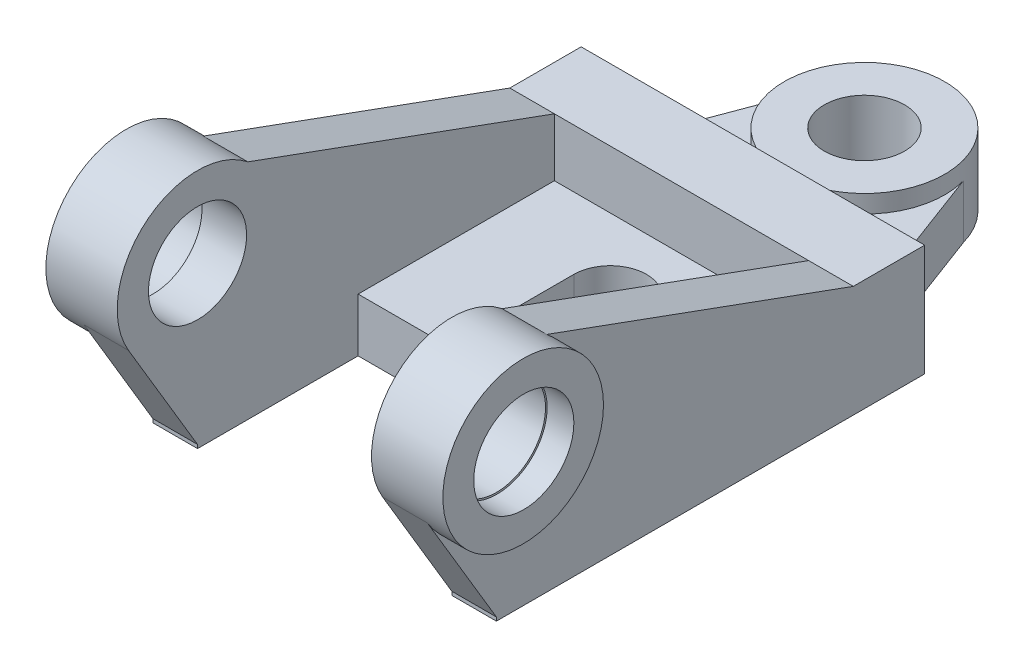
ISO-10303-21;
HEADER;
FILE_DESCRIPTION(('STEP AP214'),'2;1');
FILE_NAME('part.step','',(''),(''),'','','');
FILE_SCHEMA(('AUTOMOTIVE_DESIGN { 1 0 10303 214 1 1 1 1 }'));
ENDSEC;
DATA;
#1=APPLICATION_CONTEXT('core data for automotive mechanical design processes');
#2=APPLICATION_PROTOCOL_DEFINITION('international standard','automotive_design',2000,#1);
#3=PRODUCT_CONTEXT('',#1,'mechanical');
#4=PRODUCT('Part','Part','',(#3));
#5=PRODUCT_RELATED_PRODUCT_CATEGORY('part','',(#4));
#6=PRODUCT_DEFINITION_FORMATION('','',#4);
#7=PRODUCT_DEFINITION_CONTEXT('part definition',#1,'design');
#8=PRODUCT_DEFINITION('design','',#6,#7);
#9=PRODUCT_DEFINITION_SHAPE('','',#8);
#10=(LENGTH_UNIT() NAMED_UNIT(*) SI_UNIT(.MILLI.,.METRE.));
#11=(NAMED_UNIT(*) PLANE_ANGLE_UNIT() SI_UNIT($,.RADIAN.));
#12=(NAMED_UNIT(*) SI_UNIT($,.STERADIAN.) SOLID_ANGLE_UNIT());
#13=UNCERTAINTY_MEASURE_WITH_UNIT(LENGTH_MEASURE(1.E-05),#10,'distance_accuracy_value','');
#14=(GEOMETRIC_REPRESENTATION_CONTEXT(3) GLOBAL_UNCERTAINTY_ASSIGNED_CONTEXT((#13)) GLOBAL_UNIT_ASSIGNED_CONTEXT((#10,
#11,#12)) REPRESENTATION_CONTEXT('',''));
#15=CARTESIAN_POINT('',(0.,0.,0.));
#16=DIRECTION('',(0.,0.,1.));
#17=DIRECTION('',(1.,0.,0.));
#18=AXIS2_PLACEMENT_3D('',#15,#16,#17);
#19=CARTESIAN_POINT('',(0.,12.,0.));
#20=DIRECTION('',(0.,1.,0.));
#21=DIRECTION('',(0.,0.,1.));
#22=AXIS2_PLACEMENT_3D('',#19,#20,#21);
#23=PLANE('',#22);
#24=DIRECTION('',(0.350355850178172,0.,0.936616665581993));
#25=VECTOR('',#24,1.);
#26=CARTESIAN_POINT('',(20.6132485771023,12.,-7.71070224943851));
#27=LINE('',#26,#25);
#28=CARTESIAN_POINT('',(17.3346956287271,12.,-16.4753548986795));
#29=VERTEX_POINT('',#28);
#30=CARTESIAN_POINT('',(28.5,12.,13.3731837945135));
#31=VERTEX_POINT('',#30);
#32=EDGE_CURVE('E149',#29,#31,#27,.T.);
#33=ORIENTED_EDGE('',*,*,#32,.F.);
#34=CARTESIAN_POINT('',(0.,12.,-11.6268162054865));
#35=DIRECTION('',(0.,1.,0.));
#36=DIRECTION('',(0.,0.,1.));
#37=AXIS2_PLACEMENT_3D('',#34,#35,#36);
#38=CIRCLE('',#37,18.);
#39=CARTESIAN_POINT('',(-17.3346956287271,12.,-16.4753548986794));
#40=VERTEX_POINT('',#39);
#41=EDGE_CURVE('E147',#40,#29,#38,.T.);
#42=ORIENTED_EDGE('',*,*,#41,.F.);
#43=DIRECTION('',(0.350355850178171,0.,-0.936616665581993));
#44=VECTOR('',#43,1.);
#45=CARTESIAN_POINT('',(-20.6132485771023,12.,-7.7107022494385));
#46=LINE('',#45,#44);
#47=CARTESIAN_POINT('',(-28.5,12.,13.3731837945135));
#48=VERTEX_POINT('',#47);
#49=EDGE_CURVE('E126',#48,#40,#46,.T.);
#50=ORIENTED_EDGE('',*,*,#49,.F.);
#51=DIRECTION('',(-1.,0.,0.));
#52=VECTOR('',#51,1.);
#53=CARTESIAN_POINT('',(-38.5,12.,13.3731837945135));
#54=LINE('',#53,#52);
#55=EDGE_CURVE('E141',#31,#48,#54,.T.);
#56=ORIENTED_EDGE('',*,*,#55,.F.);
#57=EDGE_LOOP('',(#33,#42,#50,#56));
#58=FACE_BOUND('',#57,.T.);
#59=ADVANCED_FACE('F43',(#58),#23,.T.);
#60=CARTESIAN_POINT('',(-38.5,12.,0.));
#61=DIRECTION('',(1.,0.,0.));
#62=DIRECTION('',(0.,0.,-1.));
#63=AXIS2_PLACEMENT_3D('',#60,#61,#62);
#64=PLANE('',#63);
#65=CARTESIAN_POINT('',(-38.5,35.9999999975685,109.372765384346));
#66=DIRECTION('',(1.,0.,0.));
#67=DIRECTION('',(0.,0.,-1.));
#68=AXIS2_PLACEMENT_3D('',#65,#66,#67);
#69=CIRCLE('',#68,11.);
#70=CARTESIAN_POINT('',(-38.5,24.9999999975685,109.372765384346));
#71=VERTEX_POINT('',#70);
#72=CARTESIAN_POINT('',(-38.5,44.8350436191308,115.92578027866));
#73=VERTEX_POINT('',#72);
#74=EDGE_CURVE('E405',#71,#73,#69,.T.);
#75=ORIENTED_EDGE('',*,*,#74,.T.);
#76=CARTESIAN_POINT('',(-38.5,35.8172489858916,109.237217655013));
#77=DIRECTION('',(1.,0.,0.));
#78=DIRECTION('',(0.,0.,-1.));
#79=AXIS2_PLACEMENT_3D('',#76,#77,#78);
#80=CIRCLE('',#79,11.2275326811848);
#81=EDGE_CURVE('E440',#73,#73,#80,.T.);
#82=ORIENTED_EDGE('',*,*,#81,.F.);
#83=CARTESIAN_POINT('',(-38.5,24.9999999975685,109.373183794513));
#84=VERTEX_POINT('',#83);
#85=EDGE_CURVE('E403',#73,#84,#69,.T.);
#86=ORIENTED_EDGE('',*,*,#85,.T.);
#87=DIRECTION('',(0.,0.,1.));
#88=VECTOR('',#87,1.);
#89=CARTESIAN_POINT('',(-38.5,24.9999999975685,0.));
#90=LINE('',#89,#88);
#91=EDGE_CURVE('E397',#71,#84,#90,.T.);
#92=ORIENTED_EDGE('',*,*,#91,.F.);
#93=EDGE_LOOP('',(#75,#82,#86,#92));
#94=FACE_BOUND('',#93,.T.);
#95=ADVANCED_FACE('F246',(#94),#64,.F.);
#96=CARTESIAN_POINT('',(96.5,35.8172489858916,109.237217655013));
#97=DIRECTION('',(-1.,0.,0.));
#98=DIRECTION('',(0.,0.,1.));
#99=AXIS2_PLACEMENT_3D('',#96,#97,#98);
#100=CYLINDRICAL_SURFACE('',#99,11.2275326811848);
#101=CARTESIAN_POINT('',(44.5,35.8172489858916,109.237217655013));
#102=DIRECTION('',(1.,0.,0.));
#103=DIRECTION('',(0.,0.,-1.));
#104=AXIS2_PLACEMENT_3D('',#101,#102,#103);
#105=CIRCLE('',#104,11.2275326811848);
#106=CARTESIAN_POINT('',(44.5,35.8172489858916,98.0096849738277));
#107=VERTEX_POINT('',#106);
#108=EDGE_CURVE('E432',#107,#107,#105,.T.);
#109=ORIENTED_EDGE('',*,*,#108,.T.);
#110=EDGE_LOOP('',(#109));
#111=FACE_BOUND('',#110,.T.);
#112=CARTESIAN_POINT('',(38.5,35.8172489858916,109.237217655013));
#113=DIRECTION('',(-1.,0.,0.));
#114=DIRECTION('',(0.,0.,1.));
#115=AXIS2_PLACEMENT_3D('',#112,#113,#114);
#116=CIRCLE('',#115,11.2275326811848);
#117=CARTESIAN_POINT('',(38.5,44.8350436191308,115.92578027866));
#118=VERTEX_POINT('',#117);
#119=EDGE_CURVE('E11',#118,#118,#116,.F.);
#120=ORIENTED_EDGE('',*,*,#119,.F.);
#121=EDGE_LOOP('',(#120));
#122=FACE_BOUND('',#121,.T.);
#123=ADVANCED_FACE('F245',(#111,#122),#100,.F.);
#124=CARTESIAN_POINT('',(0.,12.,29.3731837945135));
#125=DIRECTION('',(0.,0.,-1.));
#126=DIRECTION('',(-1.,0.,0.));
#127=AXIS2_PLACEMENT_3D('',#124,#125,#126);
#128=PLANE('',#127);
#129=DIRECTION('',(0.,-1.,0.));
#130=VECTOR('',#129,1.);
#131=CARTESIAN_POINT('',(-28.5,0.,29.3731837945135));
#132=LINE('',#131,#130);
#133=CARTESIAN_POINT('',(-28.5,25.,29.3731837945135));
#134=VERTEX_POINT('',#133);
#135=CARTESIAN_POINT('',(-28.5,12.,29.3731837945135));
#136=VERTEX_POINT('',#135);
#137=EDGE_CURVE('E59',#134,#136,#132,.T.);
#138=ORIENTED_EDGE('',*,*,#137,.T.);
#139=DIRECTION('',(1.,0.,0.));
#140=VECTOR('',#139,1.);
#141=CARTESIAN_POINT('',(-38.5,12.,29.3731837945135));
#142=LINE('',#141,#140);
#143=CARTESIAN_POINT('',(28.5,12.,29.3731837945135));
#144=VERTEX_POINT('',#143);
#145=EDGE_CURVE('E151',#136,#144,#142,.T.);
#146=ORIENTED_EDGE('',*,*,#145,.T.);
#147=DIRECTION('',(0.,-1.,0.));
#148=VECTOR('',#147,1.);
#149=CARTESIAN_POINT('',(28.5,0.,29.3731837945135));
#150=LINE('',#149,#148);
#151=CARTESIAN_POINT('',(28.5,25.,29.3731837945135));
#152=VERTEX_POINT('',#151);
#153=EDGE_CURVE('E290',#152,#144,#150,.T.);
#154=ORIENTED_EDGE('',*,*,#153,.F.);
#155=DIRECTION('',(1.,0.,0.));
#156=VECTOR('',#155,1.);
#157=CARTESIAN_POINT('',(-38.5,25.,29.3731837945135));
#158=LINE('',#157,#156);
#159=EDGE_CURVE('E330',#134,#152,#158,.T.);
#160=ORIENTED_EDGE('',*,*,#159,.F.);
#161=EDGE_LOOP('',(#138,#146,#154,#160));
#162=FACE_BOUND('',#161,.T.);
#163=ADVANCED_FACE('F236',(#162),#128,.F.);
#164=CARTESIAN_POINT('',(0.,12.,45.3731837945135));
#165=DIRECTION('',(0.,-1.,0.));
#166=DIRECTION('',(0.,0.,-1.));
#167=AXIS2_PLACEMENT_3D('',#164,#165,#166);
#168=CYLINDRICAL_SURFACE('',#167,8.15052305771902);
#169=CARTESIAN_POINT('',(0.,0.,45.3731837945135));
#170=DIRECTION('',(0.,1.,0.));
#171=DIRECTION('',(0.,0.,1.));
#172=AXIS2_PLACEMENT_3D('',#169,#170,#171);
#173=CIRCLE('',#172,8.15052305771902);
#174=CARTESIAN_POINT('',(8.15052305771902,0.,45.3731837945135));
#175=VERTEX_POINT('',#174);
#176=CARTESIAN_POINT('',(-8.15052305771902,0.,45.3731837945135));
#177=VERTEX_POINT('',#176);
#178=EDGE_CURVE('E180',#175,#177,#173,.T.);
#179=ORIENTED_EDGE('',*,*,#178,.F.);
#180=DIRECTION('',(0.,-1.,0.));
#181=VECTOR('',#180,1.);
#182=CARTESIAN_POINT('',(8.15052305771902,12.,45.3731837945135));
#183=LINE('',#182,#181);
#184=CARTESIAN_POINT('',(8.15052305771902,12.,45.3731837945135));
#185=VERTEX_POINT('',#184);
#186=EDGE_CURVE('E107',#185,#175,#183,.T.);
#187=ORIENTED_EDGE('',*,*,#186,.F.);
#188=CARTESIAN_POINT('',(0.,12.,45.3731837945135));
#189=DIRECTION('',(0.,1.,0.));
#190=DIRECTION('',(0.,0.,1.));
#191=AXIS2_PLACEMENT_3D('',#188,#189,#190);
#192=CIRCLE('',#191,8.15052305771902);
#193=CARTESIAN_POINT('',(-8.15052305771902,12.,45.3731837945135));
#194=VERTEX_POINT('',#193);
#195=EDGE_CURVE('E162',#185,#194,#192,.T.);
#196=ORIENTED_EDGE('',*,*,#195,.T.);
#197=DIRECTION('',(0.,-1.,0.));
#198=VECTOR('',#197,1.);
#199=CARTESIAN_POINT('',(-8.15052305771902,12.,45.3731837945135));
#200=LINE('',#199,#198);
#201=EDGE_CURVE('E69',#194,#177,#200,.T.);
#202=ORIENTED_EDGE('',*,*,#201,.T.);
#203=EDGE_LOOP('',(#179,#187,#196,#202));
#204=FACE_BOUND('',#203,.T.);
#205=ADVANCED_FACE('F44',(#204),#168,.F.);
#206=CARTESIAN_POINT('',(8.15052305771903,12.,0.));
#207=DIRECTION('',(1.,0.,0.));
#208=DIRECTION('',(0.,0.,-1.));
#209=AXIS2_PLACEMENT_3D('',#206,#207,#208);
#210=PLANE('',#209);
#211=DIRECTION('',(0.,0.,1.));
#212=VECTOR('',#211,1.);
#213=CARTESIAN_POINT('',(8.15052305771903,0.,0.));
#214=LINE('',#213,#212);
#215=CARTESIAN_POINT('',(8.15052305771902,0.,73.3731837945135));
#216=VERTEX_POINT('',#215);
#217=EDGE_CURVE('E177',#175,#216,#214,.T.);
#218=ORIENTED_EDGE('',*,*,#217,.T.);
#219=DIRECTION('',(0.,-1.,0.));
#220=VECTOR('',#219,1.);
#221=CARTESIAN_POINT('',(8.15052305771902,12.,73.3731837945135));
#222=LINE('',#221,#220);
#223=CARTESIAN_POINT('',(8.15052305771902,12.,73.3731837945135));
#224=VERTEX_POINT('',#223);
#225=EDGE_CURVE('E222',#224,#216,#222,.T.);
#226=ORIENTED_EDGE('',*,*,#225,.F.);
#227=DIRECTION('',(0.,0.,1.));
#228=VECTOR('',#227,1.);
#229=CARTESIAN_POINT('',(8.15052305771903,12.,0.));
#230=LINE('',#229,#228);
#231=EDGE_CURVE('E165',#185,#224,#230,.T.);
#232=ORIENTED_EDGE('',*,*,#231,.F.);
#233=ORIENTED_EDGE('',*,*,#186,.T.);
#234=EDGE_LOOP('',(#218,#226,#232,#233));
#235=FACE_BOUND('',#234,.T.);
#236=ADVANCED_FACE('F227',(#235),#210,.F.);
#237=CARTESIAN_POINT('',(0.,12.,73.3731837945135));
#238=DIRECTION('',(0.,0.,-1.));
#239=DIRECTION('',(-1.,0.,0.));
#240=AXIS2_PLACEMENT_3D('',#237,#238,#239);
#241=PLANE('',#240);
#242=DIRECTION('',(1.,0.,0.));
#243=VECTOR('',#242,1.);
#244=CARTESIAN_POINT('',(0.,0.,73.3731837945135));
#245=LINE('',#244,#243);
#246=CARTESIAN_POINT('',(28.5,0.,73.3731837945135));
#247=VERTEX_POINT('',#246);
#248=EDGE_CURVE('E185',#216,#247,#245,.T.);
#249=ORIENTED_EDGE('',*,*,#248,.T.);
#250=DIRECTION('',(0.,-1.,0.));
#251=VECTOR('',#250,1.);
#252=CARTESIAN_POINT('',(28.5,12.,73.3731837945135));
#253=LINE('',#252,#251);
#254=CARTESIAN_POINT('',(28.5,12.,73.3731837945135));
#255=VERTEX_POINT('',#254);
#256=EDGE_CURVE('E218',#255,#247,#253,.T.);
#257=ORIENTED_EDGE('',*,*,#256,.F.);
#258=DIRECTION('',(1.,0.,0.));
#259=VECTOR('',#258,1.);
#260=CARTESIAN_POINT('',(0.,12.,73.3731837945135));
#261=LINE('',#260,#259);
#262=EDGE_CURVE('E170',#224,#255,#261,.T.);
#263=ORIENTED_EDGE('',*,*,#262,.F.);
#264=ORIENTED_EDGE('',*,*,#225,.T.);
#265=EDGE_LOOP('',(#249,#257,#263,#264));
#266=FACE_BOUND('',#265,.T.);
#267=ADVANCED_FACE('F239',(#266),#241,.F.);
#268=CARTESIAN_POINT('',(38.5,12.,0.));
#269=DIRECTION('',(1.,0.,0.));
#270=DIRECTION('',(0.,0.,-1.));
#271=AXIS2_PLACEMENT_3D('',#268,#269,#270);
#272=PLANE('',#271);
#273=CARTESIAN_POINT('',(38.5,35.9999999975685,109.372765384346));
#274=DIRECTION('',(1.,0.,0.));
#275=DIRECTION('',(0.,0.,-1.));
#276=AXIS2_PLACEMENT_3D('',#273,#274,#275);
#277=CIRCLE('',#276,18.);
#278=CARTESIAN_POINT('',(38.4999999999999,26.7927561763213,124.839719228465));
#279=VERTEX_POINT('',#278);
#280=CARTESIAN_POINT('',(38.5,50.0268956529709,98.0924197215375));
#281=VERTEX_POINT('',#280);
#282=EDGE_CURVE('E51',#279,#281,#277,.T.);
#283=ORIENTED_EDGE('',*,*,#282,.F.);
#284=DIRECTION('',(0.,0.859275213562162,0.511513545624845));
#285=VECTOR('',#284,1.);
#286=CARTESIAN_POINT('',(38.5,-47.860695182119,80.3996481141306));
#287=LINE('',#286,#285);
#288=CARTESIAN_POINT('',(38.5,0.811018934463448,109.373183794513));
#289=VERTEX_POINT('',#288);
#290=EDGE_CURVE('E351',#289,#279,#287,.T.);
#291=ORIENTED_EDGE('',*,*,#290,.F.);
#292=DIRECTION('',(0.,1.,0.));
#293=VECTOR('',#292,1.);
#294=CARTESIAN_POINT('',(38.5,0.,109.373183794513));
#295=LINE('',#294,#293);
#296=CARTESIAN_POINT('',(38.5,0.,109.373183794513));
#297=VERTEX_POINT('',#296);
#298=EDGE_CURVE('E349',#297,#289,#295,.T.);
#299=ORIENTED_EDGE('',*,*,#298,.F.);
#300=DIRECTION('',(0.,0.,1.));
#301=VECTOR('',#300,1.);
#302=CARTESIAN_POINT('',(38.5,0.,0.));
#303=LINE('',#302,#301);
#304=CARTESIAN_POINT('',(38.5,0.,13.3731837945135));
#305=VERTEX_POINT('',#304);
#306=EDGE_CURVE('E184',#305,#297,#303,.T.);
#307=ORIENTED_EDGE('',*,*,#306,.F.);
#308=DIRECTION('',(0.,-1.,0.));
#309=VECTOR('',#308,1.);
#310=CARTESIAN_POINT('',(38.5,12.,13.3731837945135));
#311=LINE('',#310,#309);
#312=CARTESIAN_POINT('',(38.5,25.,13.3731837945135));
#313=VERTEX_POINT('',#312);
#314=EDGE_CURVE('E220',#313,#305,#311,.T.);
#315=ORIENTED_EDGE('',*,*,#314,.F.);
#316=DIRECTION('',(0.,0.,-1.));
#317=VECTOR('',#316,1.);
#318=CARTESIAN_POINT('',(38.5,25.,13.3731837945135));
#319=LINE('',#318,#317);
#320=CARTESIAN_POINT('',(38.5,25.,29.3731837945135));
#321=VERTEX_POINT('',#320);
#322=EDGE_CURVE('E325',#321,#313,#319,.T.);
#323=ORIENTED_EDGE('',*,*,#322,.F.);
#324=DIRECTION('',(0.,0.342202927058115,0.939626072814531));
#325=VECTOR('',#324,1.);
#326=CARTESIAN_POINT('',(38.5,12.6276933750267,-4.59888647191619));
#327=LINE('',#326,#325);
#328=EDGE_CURVE('E353',#321,#281,#327,.T.);
#329=ORIENTED_EDGE('',*,*,#328,.T.);
#330=EDGE_LOOP('',(#283,#291,#299,#307,#315,#323,#329));
#331=FACE_BOUND('',#330,.T.);
#332=ADVANCED_FACE('F699',(#331),#272,.T.);
#333=CARTESIAN_POINT('',(20.6132485771023,12.,-7.71070224943851));
#334=DIRECTION('',(0.936616665581993,0.,-0.350355850178172));
#335=DIRECTION('',(-0.350355850178172,0.,-0.936616665581993));
#336=AXIS2_PLACEMENT_3D('',#333,#334,#335);
#337=PLANE('',#336);
#338=DIRECTION('',(0.350355850178172,0.,0.936616665581993));
#339=VECTOR('',#338,1.);
#340=CARTESIAN_POINT('',(20.6132485771023,0.,-7.71070224943851));
#341=LINE('',#340,#339);
#342=CARTESIAN_POINT('',(17.3346956287271,0.,-16.4753548986795));
#343=VERTEX_POINT('',#342);
#344=CARTESIAN_POINT('',(28.5,0.,13.3731837945135));
#345=VERTEX_POINT('',#344);
#346=EDGE_CURVE('E192',#343,#345,#341,.T.);
#347=ORIENTED_EDGE('',*,*,#346,.F.);
#348=DIRECTION('',(0.,-1.,0.));
#349=VECTOR('',#348,1.);
#350=CARTESIAN_POINT('',(17.3346956287271,12.,-16.4753548986795));
#351=LINE('',#350,#349);
#352=EDGE_CURVE('E213',#29,#343,#351,.T.);
#353=ORIENTED_EDGE('',*,*,#352,.F.);
#354=ORIENTED_EDGE('',*,*,#32,.T.);
#355=DIRECTION('',(0.,-1.,0.));
#356=VECTOR('',#355,1.);
#357=CARTESIAN_POINT('',(28.5,12.,13.3731837945135));
#358=LINE('',#357,#356);
#359=EDGE_CURVE('E154',#31,#345,#358,.T.);
#360=ORIENTED_EDGE('',*,*,#359,.T.);
#361=EDGE_LOOP('',(#347,#353,#354,#360));
#362=FACE_BOUND('',#361,.T.);
#363=ADVANCED_FACE('F681',(#362),#337,.T.);
#364=CARTESIAN_POINT('',(0.,12.,-11.6268162054865));
#365=DIRECTION('',(0.,-1.,0.));
#366=DIRECTION('',(0.,0.,-1.));
#367=AXIS2_PLACEMENT_3D('',#364,#365,#366);
#368=CYLINDRICAL_SURFACE('',#367,18.);
#369=CARTESIAN_POINT('',(0.,0.,-11.6268162054865));
#370=DIRECTION('',(0.,1.,0.));
#371=DIRECTION('',(0.,0.,1.));
#372=AXIS2_PLACEMENT_3D('',#369,#370,#371);
#373=CIRCLE('',#372,18.);
#374=CARTESIAN_POINT('',(-17.3346956287271,0.,-16.4753548986795));
#375=VERTEX_POINT('',#374);
#376=EDGE_CURVE('E193',#343,#375,#373,.T.);
#377=ORIENTED_EDGE('',*,*,#376,.T.);
#378=DIRECTION('',(0.,-1.,0.));
#379=VECTOR('',#378,1.);
#380=CARTESIAN_POINT('',(-17.3346956287271,12.,-16.4753548986795));
#381=LINE('',#380,#379);
#382=EDGE_CURVE('E140',#40,#375,#381,.T.);
#383=ORIENTED_EDGE('',*,*,#382,.F.);
#384=ORIENTED_EDGE('',*,*,#41,.T.);
#385=ORIENTED_EDGE('',*,*,#352,.T.);
#386=EDGE_LOOP('',(#377,#383,#384,#385));
#387=FACE_BOUND('',#386,.T.);
#388=CARTESIAN_POINT('',(0.,16.,-11.6268162054865));
#389=DIRECTION('',(0.,1.,0.));
#390=DIRECTION('',(0.,0.,1.));
#391=AXIS2_PLACEMENT_3D('',#388,#389,#390);
#392=CIRCLE('',#391,18.);
#393=CARTESIAN_POINT('',(0.,16.,6.37318379451345));
#394=VERTEX_POINT('',#393);
#395=EDGE_CURVE('E470',#394,#394,#392,.T.);
#396=ORIENTED_EDGE('',*,*,#395,.F.);
#397=EDGE_LOOP('',(#396));
#398=FACE_BOUND('',#397,.T.);
#399=ADVANCED_FACE('F678',(#387,#398),#368,.T.);
#400=CARTESIAN_POINT('',(-20.6132485771023,12.,-7.7107022494385));
#401=DIRECTION('',(-0.936616665581993,0.,-0.350355850178171));
#402=DIRECTION('',(-0.350355850178171,0.,0.936616665581993));
#403=AXIS2_PLACEMENT_3D('',#400,#401,#402);
#404=PLANE('',#403);
#405=DIRECTION('',(0.350355850178171,0.,-0.936616665581993));
#406=VECTOR('',#405,1.);
#407=CARTESIAN_POINT('',(-20.6132485771023,0.,-7.7107022494385));
#408=LINE('',#407,#406);
#409=CARTESIAN_POINT('',(-28.5,0.,13.3731837945135));
#410=VERTEX_POINT('',#409);
#411=EDGE_CURVE('E134',#410,#375,#408,.T.);
#412=ORIENTED_EDGE('',*,*,#411,.F.);
#413=DIRECTION('',(0.,-1.,0.));
#414=VECTOR('',#413,1.);
#415=CARTESIAN_POINT('',(-28.5,12.,13.3731837945135));
#416=LINE('',#415,#414);
#417=EDGE_CURVE('E123',#48,#410,#416,.T.);
#418=ORIENTED_EDGE('',*,*,#417,.F.);
#419=ORIENTED_EDGE('',*,*,#49,.T.);
#420=ORIENTED_EDGE('',*,*,#382,.T.);
#421=EDGE_LOOP('',(#412,#418,#419,#420));
#422=FACE_BOUND('',#421,.T.);
#423=ADVANCED_FACE('F130',(#422),#404,.T.);
#424=CARTESIAN_POINT('',(0.,12.,13.3731837945135));
#425=DIRECTION('',(0.,0.,-1.));
#426=DIRECTION('',(-1.,0.,0.));
#427=AXIS2_PLACEMENT_3D('',#424,#425,#426);
#428=PLANE('',#427);
#429=DIRECTION('',(1.,0.,0.));
#430=VECTOR('',#429,1.);
#431=CARTESIAN_POINT('',(0.,0.,13.3731837945135));
#432=LINE('',#431,#430);
#433=CARTESIAN_POINT('',(-38.5,0.,13.3731837945135));
#434=VERTEX_POINT('',#433);
#435=EDGE_CURVE('E195',#434,#410,#432,.T.);
#436=ORIENTED_EDGE('',*,*,#435,.F.);
#437=DIRECTION('',(0.,-1.,0.));
#438=VECTOR('',#437,1.);
#439=CARTESIAN_POINT('',(-38.5,12.,13.3731837945135));
#440=LINE('',#439,#438);
#441=CARTESIAN_POINT('',(-38.5,25.,13.3731837945135));
#442=VERTEX_POINT('',#441);
#443=EDGE_CURVE('E137',#442,#434,#440,.T.);
#444=ORIENTED_EDGE('',*,*,#443,.F.);
#445=DIRECTION('',(-1.,0.,0.));
#446=VECTOR('',#445,1.);
#447=CARTESIAN_POINT('',(-38.5,25.,13.3731837945135));
#448=LINE('',#447,#446);
#449=EDGE_CURVE('E179',#313,#442,#448,.T.);
#450=ORIENTED_EDGE('',*,*,#449,.F.);
#451=ORIENTED_EDGE('',*,*,#314,.T.);
#452=EDGE_CURVE('E189',#345,#305,#432,.T.);
#453=ORIENTED_EDGE('',*,*,#452,.F.);
#454=ORIENTED_EDGE('',*,*,#359,.F.);
#455=ORIENTED_EDGE('',*,*,#55,.T.);
#456=ORIENTED_EDGE('',*,*,#417,.T.);
#457=EDGE_LOOP('',(#436,#444,#450,#451,#453,#454,#455,#456));
#458=FACE_BOUND('',#457,.T.);
#459=ADVANCED_FACE('F148',(#458),#428,.T.);
#460=DIRECTION('',(0.,0.859275213562162,0.511513545624845));
#461=VECTOR('',#460,1.);
#462=CARTESIAN_POINT('',(-38.5,-47.860695182119,80.3996481141306));
#463=LINE('',#462,#461);
#464=CARTESIAN_POINT('',(-38.5,0.811018934463448,109.373183794513));
#465=VERTEX_POINT('',#464);
#466=CARTESIAN_POINT('',(-38.4999999999999,26.7927561763213,124.839719228465));
#467=VERTEX_POINT('',#466);
#468=EDGE_CURVE('E406',#465,#467,#463,.T.);
#469=ORIENTED_EDGE('',*,*,#468,.T.);
#470=CARTESIAN_POINT('',(-38.5,35.9999999975685,109.372765384346));
#471=DIRECTION('',(1.,0.,0.));
#472=DIRECTION('',(0.,0.,-1.));
#473=AXIS2_PLACEMENT_3D('',#470,#471,#472);
#474=CIRCLE('',#473,18.);
#475=CARTESIAN_POINT('',(-38.5,50.0268956557217,98.0924197264698));
#476=VERTEX_POINT('',#475);
#477=EDGE_CURVE('E439',#467,#476,#474,.T.);
#478=ORIENTED_EDGE('',*,*,#477,.T.);
#479=DIRECTION('',(0.,0.342202927058115,0.939626072814531));
#480=VECTOR('',#479,1.);
#481=CARTESIAN_POINT('',(-38.5,12.6276933750267,-4.59888647191619));
#482=LINE('',#481,#480);
#483=CARTESIAN_POINT('',(-38.5,25.,29.3731837945135));
#484=VERTEX_POINT('',#483);
#485=EDGE_CURVE('E329',#484,#476,#482,.T.);
#486=ORIENTED_EDGE('',*,*,#485,.F.);
#487=DIRECTION('',(0.,0.,1.));
#488=VECTOR('',#487,1.);
#489=CARTESIAN_POINT('',(-38.5,25.,13.3731837945135));
#490=LINE('',#489,#488);
#491=EDGE_CURVE('E318',#442,#484,#490,.T.);
#492=ORIENTED_EDGE('',*,*,#491,.F.);
#493=ORIENTED_EDGE('',*,*,#443,.T.);
#494=DIRECTION('',(0.,0.,1.));
#495=VECTOR('',#494,1.);
#496=CARTESIAN_POINT('',(-38.5,0.,0.));
#497=LINE('',#496,#495);
#498=CARTESIAN_POINT('',(-38.5,0.,109.373183794513));
#499=VERTEX_POINT('',#498);
#500=EDGE_CURVE('E196',#434,#499,#497,.T.);
#501=ORIENTED_EDGE('',*,*,#500,.T.);
#502=DIRECTION('',(0.,1.,0.));
#503=VECTOR('',#502,1.);
#504=CARTESIAN_POINT('',(-38.5,0.,109.373183794513));
#505=LINE('',#504,#503);
#506=EDGE_CURVE('E407',#499,#465,#505,.T.);
#507=ORIENTED_EDGE('',*,*,#506,.T.);
#508=EDGE_LOOP('',(#469,#478,#486,#492,#493,#501,#507));
#509=FACE_BOUND('',#508,.T.);
#510=ADVANCED_FACE('F257',(#509),#64,.F.);
#511=CARTESIAN_POINT('',(0.,12.,73.3731837945135));
#512=DIRECTION('',(0.,0.,-1.));
#513=DIRECTION('',(-1.,0.,0.));
#514=AXIS2_PLACEMENT_3D('',#511,#512,#513);
#515=PLANE('',#514);
#516=DIRECTION('',(1.,0.,0.));
#517=VECTOR('',#516,1.);
#518=CARTESIAN_POINT('',(0.,0.,73.3731837945135));
#519=LINE('',#518,#517);
#520=CARTESIAN_POINT('',(-28.5,0.,73.3731837945135));
#521=VERTEX_POINT('',#520);
#522=CARTESIAN_POINT('',(-8.15052305771903,0.,73.3731837945135));
#523=VERTEX_POINT('',#522);
#524=EDGE_CURVE('E205',#521,#523,#519,.T.);
#525=ORIENTED_EDGE('',*,*,#524,.T.);
#526=DIRECTION('',(0.,-1.,0.));
#527=VECTOR('',#526,1.);
#528=CARTESIAN_POINT('',(-8.15052305771903,12.,73.3731837945135));
#529=LINE('',#528,#527);
#530=CARTESIAN_POINT('',(-8.15052305771903,12.,73.3731837945135));
#531=VERTEX_POINT('',#530);
#532=EDGE_CURVE('E212',#531,#523,#529,.T.);
#533=ORIENTED_EDGE('',*,*,#532,.F.);
#534=DIRECTION('',(1.,0.,0.));
#535=VECTOR('',#534,1.);
#536=CARTESIAN_POINT('',(0.,12.,73.3731837945135));
#537=LINE('',#536,#535);
#538=CARTESIAN_POINT('',(-28.5,12.,73.3731837945135));
#539=VERTEX_POINT('',#538);
#540=EDGE_CURVE('E150',#539,#531,#537,.T.);
#541=ORIENTED_EDGE('',*,*,#540,.F.);
#542=DIRECTION('',(0.,-1.,0.));
#543=VECTOR('',#542,1.);
#544=CARTESIAN_POINT('',(-28.5,12.,73.3731837945135));
#545=LINE('',#544,#543);
#546=EDGE_CURVE('E357',#539,#521,#545,.T.);
#547=ORIENTED_EDGE('',*,*,#546,.T.);
#548=EDGE_LOOP('',(#525,#533,#541,#547));
#549=FACE_BOUND('',#548,.T.);
#550=ADVANCED_FACE('F597',(#549),#515,.F.);
#551=CARTESIAN_POINT('',(-8.15052305771901,12.,0.));
#552=DIRECTION('',(1.,0.,0.));
#553=DIRECTION('',(0.,0.,-1.));
#554=AXIS2_PLACEMENT_3D('',#551,#552,#553);
#555=PLANE('',#554);
#556=DIRECTION('',(0.,0.,1.));
#557=VECTOR('',#556,1.);
#558=CARTESIAN_POINT('',(-8.15052305771901,0.,0.));
#559=LINE('',#558,#557);
#560=EDGE_CURVE('E204',#177,#523,#559,.T.);
#561=ORIENTED_EDGE('',*,*,#560,.F.);
#562=ORIENTED_EDGE('',*,*,#201,.F.);
#563=DIRECTION('',(0.,0.,1.));
#564=VECTOR('',#563,1.);
#565=CARTESIAN_POINT('',(-8.15052305771901,12.,0.));
#566=LINE('',#565,#564);
#567=EDGE_CURVE('E174',#194,#531,#566,.T.);
#568=ORIENTED_EDGE('',*,*,#567,.T.);
#569=ORIENTED_EDGE('',*,*,#532,.T.);
#570=EDGE_LOOP('',(#561,#562,#568,#569));
#571=FACE_BOUND('',#570,.T.);
#572=ADVANCED_FACE('F268',(#571),#555,.T.);
#573=CARTESIAN_POINT('',(0.,12.,-11.6268162054865));
#574=DIRECTION('',(0.,-1.,0.));
#575=DIRECTION('',(0.,0.,-1.));
#576=AXIS2_PLACEMENT_3D('',#573,#574,#575);
#577=CYLINDRICAL_SURFACE('',#576,9.);
#578=CARTESIAN_POINT('',(0.,0.,-11.6268162054865));
#579=DIRECTION('',(0.,1.,0.));
#580=DIRECTION('',(0.,0.,1.));
#581=AXIS2_PLACEMENT_3D('',#578,#579,#580);
#582=CIRCLE('',#581,9.);
#583=CARTESIAN_POINT('',(0.,0.,-2.62681620548655));
#584=VERTEX_POINT('',#583);
#585=EDGE_CURVE('E164',#584,#584,#582,.T.);
#586=ORIENTED_EDGE('',*,*,#585,.F.);
#587=EDGE_LOOP('',(#586));
#588=FACE_BOUND('',#587,.T.);
#589=CARTESIAN_POINT('',(0.,16.,-11.6268162054865));
#590=DIRECTION('',(0.,1.,0.));
#591=DIRECTION('',(0.,0.,1.));
#592=AXIS2_PLACEMENT_3D('',#589,#590,#591);
#593=CIRCLE('',#592,9.);
#594=CARTESIAN_POINT('',(0.,16.,-2.62681620548655));
#595=VERTEX_POINT('',#594);
#596=EDGE_CURVE('E469',#595,#595,#593,.T.);
#597=ORIENTED_EDGE('',*,*,#596,.T.);
#598=EDGE_LOOP('',(#597));
#599=FACE_BOUND('',#598,.T.);
#600=ADVANCED_FACE('F258',(#588,#599),#577,.F.);
#601=ORIENTED_EDGE('',*,*,#145,.F.);
#602=DIRECTION('',(0.,0.,1.));
#603=VECTOR('',#602,1.);
#604=CARTESIAN_POINT('',(-28.5,12.,0.));
#605=LINE('',#604,#603);
#606=EDGE_CURVE('E280',#136,#539,#605,.T.);
#607=ORIENTED_EDGE('',*,*,#606,.T.);
#608=ORIENTED_EDGE('',*,*,#540,.T.);
#609=ORIENTED_EDGE('',*,*,#567,.F.);
#610=ORIENTED_EDGE('',*,*,#195,.F.);
#611=ORIENTED_EDGE('',*,*,#231,.T.);
#612=ORIENTED_EDGE('',*,*,#262,.T.);
#613=DIRECTION('',(0.,0.,1.));
#614=VECTOR('',#613,1.);
#615=CARTESIAN_POINT('',(28.5,12.,0.));
#616=LINE('',#615,#614);
#617=EDGE_CURVE('E167',#144,#255,#616,.T.);
#618=ORIENTED_EDGE('',*,*,#617,.F.);
#619=EDGE_LOOP('',(#601,#607,#608,#609,#610,#611,#612,#618));
#620=FACE_BOUND('',#619,.T.);
#621=ADVANCED_FACE('F247',(#620),#23,.T.);
#622=CARTESIAN_POINT('',(0.,0.,0.));
#623=DIRECTION('',(0.,1.,0.));
#624=DIRECTION('',(0.,0.,1.));
#625=AXIS2_PLACEMENT_3D('',#622,#623,#624);
#626=PLANE('',#625);
#627=ORIENTED_EDGE('',*,*,#306,.T.);
#628=DIRECTION('',(1.,0.,0.));
#629=VECTOR('',#628,1.);
#630=CARTESIAN_POINT('',(28.5,0.,109.373183794513));
#631=LINE('',#630,#629);
#632=CARTESIAN_POINT('',(28.5,0.,109.373183794513));
#633=VERTEX_POINT('',#632);
#634=EDGE_CURVE('E335',#633,#297,#631,.T.);
#635=ORIENTED_EDGE('',*,*,#634,.F.);
#636=DIRECTION('',(0.,0.,1.));
#637=VECTOR('',#636,1.);
#638=CARTESIAN_POINT('',(28.5,0.,0.));
#639=LINE('',#638,#637);
#640=EDGE_CURVE('E360',#247,#633,#639,.T.);
#641=ORIENTED_EDGE('',*,*,#640,.F.);
#642=ORIENTED_EDGE('',*,*,#248,.F.);
#643=ORIENTED_EDGE('',*,*,#217,.F.);
#644=ORIENTED_EDGE('',*,*,#178,.T.);
#645=ORIENTED_EDGE('',*,*,#560,.T.);
#646=ORIENTED_EDGE('',*,*,#524,.F.);
#647=DIRECTION('',(0.,0.,1.));
#648=VECTOR('',#647,1.);
#649=CARTESIAN_POINT('',(-28.5,0.,0.));
#650=LINE('',#649,#648);
#651=CARTESIAN_POINT('',(-28.5,0.,109.373183794513));
#652=VERTEX_POINT('',#651);
#653=EDGE_CURVE('E418',#521,#652,#650,.T.);
#654=ORIENTED_EDGE('',*,*,#653,.T.);
#655=DIRECTION('',(-1.,0.,0.));
#656=VECTOR('',#655,1.);
#657=CARTESIAN_POINT('',(-28.5,0.,109.373183794513));
#658=LINE('',#657,#656);
#659=EDGE_CURVE('E390',#652,#499,#658,.T.);
#660=ORIENTED_EDGE('',*,*,#659,.T.);
#661=ORIENTED_EDGE('',*,*,#500,.F.);
#662=ORIENTED_EDGE('',*,*,#435,.T.);
#663=ORIENTED_EDGE('',*,*,#411,.T.);
#664=ORIENTED_EDGE('',*,*,#376,.F.);
#665=ORIENTED_EDGE('',*,*,#346,.T.);
#666=ORIENTED_EDGE('',*,*,#452,.T.);
#667=EDGE_LOOP('',(#627,#635,#641,#642,#643,#644,#645,#646,#654,#660,#661,#662,#663,#664,#665,#666));
#668=FACE_BOUND('',#667,.T.);
#669=ORIENTED_EDGE('',*,*,#585,.T.);
#670=EDGE_LOOP('',(#669));
#671=FACE_BOUND('',#670,.T.);
#672=ADVANCED_FACE('F235',(#668,#671),#626,.F.);
#673=CARTESIAN_POINT('',(0.,25.,0.));
#674=DIRECTION('',(0.,1.,0.));
#675=DIRECTION('',(0.,0.,1.));
#676=AXIS2_PLACEMENT_3D('',#673,#674,#675);
#677=PLANE('',#676);
#678=ORIENTED_EDGE('',*,*,#491,.T.);
#679=DIRECTION('',(-1.,0.,0.));
#680=VECTOR('',#679,1.);
#681=CARTESIAN_POINT('',(-28.5,25.,29.3731837945135));
#682=LINE('',#681,#680);
#683=EDGE_CURVE('E388',#134,#484,#682,.T.);
#684=ORIENTED_EDGE('',*,*,#683,.F.);
#685=ORIENTED_EDGE('',*,*,#159,.T.);
#686=DIRECTION('',(1.,0.,0.));
#687=VECTOR('',#686,1.);
#688=CARTESIAN_POINT('',(28.5,25.,29.3731837945135));
#689=LINE('',#688,#687);
#690=EDGE_CURVE('E326',#152,#321,#689,.T.);
#691=ORIENTED_EDGE('',*,*,#690,.T.);
#692=ORIENTED_EDGE('',*,*,#322,.T.);
#693=ORIENTED_EDGE('',*,*,#449,.T.);
#694=EDGE_LOOP('',(#678,#684,#685,#691,#692,#693));
#695=FACE_BOUND('',#694,.T.);
#696=ADVANCED_FACE('F270',(#695),#677,.T.);
#697=CARTESIAN_POINT('',(28.5,0.,0.));
#698=DIRECTION('',(1.,0.,0.));
#699=DIRECTION('',(0.,0.,-1.));
#700=AXIS2_PLACEMENT_3D('',#697,#698,#699);
#701=PLANE('',#700);
#702=CARTESIAN_POINT('',(28.5,35.9999999975685,109.372765384346));
#703=DIRECTION('',(1.,0.,0.));
#704=DIRECTION('',(0.,0.,-1.));
#705=AXIS2_PLACEMENT_3D('',#702,#703,#704);
#706=CIRCLE('',#705,11.);
#707=CARTESIAN_POINT('',(28.5,24.9999999975685,109.372765384346));
#708=VERTEX_POINT('',#707);
#709=CARTESIAN_POINT('',(28.5,24.9999999975685,109.373183794513));
#710=VERTEX_POINT('',#709);
#711=EDGE_CURVE('E452',#708,#710,#706,.T.);
#712=ORIENTED_EDGE('',*,*,#711,.T.);
#713=DIRECTION('',(0.,0.,1.));
#714=VECTOR('',#713,1.);
#715=CARTESIAN_POINT('',(28.5,24.9999999975685,0.));
#716=LINE('',#715,#714);
#717=EDGE_CURVE('E444',#708,#710,#716,.T.);
#718=ORIENTED_EDGE('',*,*,#717,.F.);
#719=EDGE_LOOP('',(#712,#718));
#720=FACE_BOUND('',#719,.T.);
#721=ORIENTED_EDGE('',*,*,#617,.T.);
#722=ORIENTED_EDGE('',*,*,#256,.T.);
#723=ORIENTED_EDGE('',*,*,#640,.T.);
#724=DIRECTION('',(0.,1.,0.));
#725=VECTOR('',#724,1.);
#726=CARTESIAN_POINT('',(28.5,0.,109.373183794513));
#727=LINE('',#726,#725);
#728=CARTESIAN_POINT('',(28.5,0.811018934463448,109.373183794513));
#729=VERTEX_POINT('',#728);
#730=EDGE_CURVE('E365',#633,#729,#727,.T.);
#731=ORIENTED_EDGE('',*,*,#730,.T.);
#732=DIRECTION('',(0.,0.859275213562162,0.511513545624845));
#733=VECTOR('',#732,1.);
#734=CARTESIAN_POINT('',(28.5,-47.860695182119,80.3996481141306));
#735=LINE('',#734,#733);
#736=CARTESIAN_POINT('',(28.5,26.7927561763213,124.839719228465));
#737=VERTEX_POINT('',#736);
#738=EDGE_CURVE('E362',#729,#737,#735,.T.);
#739=ORIENTED_EDGE('',*,*,#738,.T.);
#740=CARTESIAN_POINT('',(28.5,35.9999999975685,109.372765384346));
#741=DIRECTION('',(1.,0.,0.));
#742=DIRECTION('',(0.,0.,-1.));
#743=AXIS2_PLACEMENT_3D('',#740,#741,#742);
#744=CIRCLE('',#743,18.);
#745=CARTESIAN_POINT('',(28.5,50.0268956557217,98.0924197264698));
#746=VERTEX_POINT('',#745);
#747=EDGE_CURVE('E368',#746,#737,#744,.T.);
#748=ORIENTED_EDGE('',*,*,#747,.F.);
#749=DIRECTION('',(0.,0.342202927058115,0.939626072814531));
#750=VECTOR('',#749,1.);
#751=CARTESIAN_POINT('',(28.5,12.6276933750267,-4.5988864719162));
#752=LINE('',#751,#750);
#753=EDGE_CURVE('E348',#152,#746,#752,.T.);
#754=ORIENTED_EDGE('',*,*,#753,.F.);
#755=ORIENTED_EDGE('',*,*,#153,.T.);
#756=EDGE_LOOP('',(#721,#722,#723,#731,#739,#748,#754,#755));
#757=FACE_BOUND('',#756,.T.);
#758=ADVANCED_FACE('F539',(#720,#757),#701,.F.);
#759=CARTESIAN_POINT('',(28.5,12.6276933750267,-4.5988864719162));
#760=DIRECTION('',(0.,0.939626072814531,-0.342202927058115));
#761=DIRECTION('',(0.,0.342202927058115,0.939626072814531));
#762=AXIS2_PLACEMENT_3D('',#759,#760,#761);
#763=PLANE('',#762);
#764=ORIENTED_EDGE('',*,*,#328,.F.);
#765=ORIENTED_EDGE('',*,*,#690,.F.);
#766=ORIENTED_EDGE('',*,*,#753,.T.);
#767=DIRECTION('',(1.,0.,0.));
#768=VECTOR('',#767,1.);
#769=CARTESIAN_POINT('',(28.5,50.0268956557217,98.0924197264698));
#770=LINE('',#769,#768);
#771=EDGE_CURVE('E334',#746,#281,#770,.T.);
#772=ORIENTED_EDGE('',*,*,#771,.T.);
#773=EDGE_LOOP('',(#764,#765,#766,#772));
#774=FACE_BOUND('',#773,.T.);
#775=ADVANCED_FACE('F542',(#774),#763,.T.);
#776=CARTESIAN_POINT('',(28.5,0.,109.373183794513));
#777=DIRECTION('',(0.,0.,-1.));
#778=DIRECTION('',(-1.,0.,0.));
#779=AXIS2_PLACEMENT_3D('',#776,#777,#778);
#780=PLANE('',#779);
#781=ORIENTED_EDGE('',*,*,#298,.T.);
#782=DIRECTION('',(1.,0.,0.));
#783=VECTOR('',#782,1.);
#784=CARTESIAN_POINT('',(28.5,0.811018934463448,109.373183794513));
#785=LINE('',#784,#783);
#786=EDGE_CURVE('E345',#729,#289,#785,.T.);
#787=ORIENTED_EDGE('',*,*,#786,.F.);
#788=ORIENTED_EDGE('',*,*,#730,.F.);
#789=ORIENTED_EDGE('',*,*,#634,.T.);
#790=EDGE_LOOP('',(#781,#787,#788,#789));
#791=FACE_BOUND('',#790,.T.);
#792=ADVANCED_FACE('F545',(#791),#780,.F.);
#793=CARTESIAN_POINT('',(28.5,-47.860695182119,80.3996481141306));
#794=DIRECTION('',(0.,0.511513545624845,-0.859275213562162));
#795=DIRECTION('',(0.,0.859275213562162,0.511513545624845));
#796=AXIS2_PLACEMENT_3D('',#793,#794,#795);
#797=PLANE('',#796);
#798=ORIENTED_EDGE('',*,*,#290,.T.);
#799=DIRECTION('',(1.,0.,0.));
#800=VECTOR('',#799,1.);
#801=CARTESIAN_POINT('',(28.5,26.7927561763213,124.839719228465));
#802=LINE('',#801,#800);
#803=EDGE_CURVE('E339',#737,#279,#802,.T.);
#804=ORIENTED_EDGE('',*,*,#803,.F.);
#805=ORIENTED_EDGE('',*,*,#738,.F.);
#806=ORIENTED_EDGE('',*,*,#786,.T.);
#807=EDGE_LOOP('',(#798,#804,#805,#806));
#808=FACE_BOUND('',#807,.T.);
#809=ADVANCED_FACE('F546',(#808),#797,.F.);
#810=CARTESIAN_POINT('',(28.5,35.9999999975685,109.372765384346));
#811=DIRECTION('',(1.,0.,0.));
#812=DIRECTION('',(0.,0.,-1.));
#813=AXIS2_PLACEMENT_3D('',#810,#811,#812);
#814=CYLINDRICAL_SURFACE('',#813,18.);
#815=ORIENTED_EDGE('',*,*,#803,.T.);
#816=ORIENTED_EDGE('',*,*,#282,.T.);
#817=ORIENTED_EDGE('',*,*,#771,.F.);
#818=ORIENTED_EDGE('',*,*,#747,.T.);
#819=EDGE_LOOP('',(#815,#816,#817,#818));
#820=FACE_BOUND('',#819,.T.);
#821=CARTESIAN_POINT('',(44.5,35.9999999975685,109.372765384346));
#822=DIRECTION('',(1.,0.,0.));
#823=DIRECTION('',(0.,0.,-1.));
#824=AXIS2_PLACEMENT_3D('',#821,#822,#823);
#825=CIRCLE('',#824,18.);
#826=CARTESIAN_POINT('',(44.5,35.9999999975685,91.3727653843465));
#827=VERTEX_POINT('',#826);
#828=EDGE_CURVE('E414',#827,#827,#825,.T.);
#829=ORIENTED_EDGE('',*,*,#828,.F.);
#830=EDGE_LOOP('',(#829));
#831=FACE_BOUND('',#830,.T.);
#832=ADVANCED_FACE('F511',(#820,#831),#814,.T.);
#833=CARTESIAN_POINT('',(-28.5,0.,0.));
#834=DIRECTION('',(-1.,0.,0.));
#835=DIRECTION('',(0.,0.,-1.));
#836=AXIS2_PLACEMENT_3D('',#833,#834,#835);
#837=PLANE('',#836);
#838=DIRECTION('',(0.,0.,1.));
#839=VECTOR('',#838,1.);
#840=CARTESIAN_POINT('',(-28.5,24.9999999975685,0.));
#841=LINE('',#840,#839);
#842=CARTESIAN_POINT('',(-28.5,24.9999999975685,109.372765384346));
#843=VERTEX_POINT('',#842);
#844=CARTESIAN_POINT('',(-28.5,24.9999999975685,109.373183794513));
#845=VERTEX_POINT('',#844);
#846=EDGE_CURVE('E382',#843,#845,#841,.T.);
#847=ORIENTED_EDGE('',*,*,#846,.T.);
#848=CARTESIAN_POINT('',(-28.5,35.9999999975685,109.372765384346));
#849=DIRECTION('',(1.,0.,0.));
#850=DIRECTION('',(0.,0.,-1.));
#851=AXIS2_PLACEMENT_3D('',#848,#849,#850);
#852=CIRCLE('',#851,11.);
#853=EDGE_CURVE('E413',#843,#845,#852,.T.);
#854=ORIENTED_EDGE('',*,*,#853,.F.);
#855=EDGE_LOOP('',(#847,#854));
#856=FACE_BOUND('',#855,.T.);
#857=ORIENTED_EDGE('',*,*,#606,.F.);
#858=ORIENTED_EDGE('',*,*,#137,.F.);
#859=DIRECTION('',(0.,0.342202927058115,0.939626072814531));
#860=VECTOR('',#859,1.);
#861=CARTESIAN_POINT('',(-28.5,12.6276933750267,-4.5988864719162));
#862=LINE('',#861,#860);
#863=CARTESIAN_POINT('',(-28.5,50.0268956557217,98.0924197264698));
#864=VERTEX_POINT('',#863);
#865=EDGE_CURVE('E402',#134,#864,#862,.T.);
#866=ORIENTED_EDGE('',*,*,#865,.T.);
#867=CARTESIAN_POINT('',(-28.5,35.9999999975685,109.372765384346));
#868=DIRECTION('',(1.,0.,0.));
#869=DIRECTION('',(0.,0.,-1.));
#870=AXIS2_PLACEMENT_3D('',#867,#868,#869);
#871=CIRCLE('',#870,18.);
#872=CARTESIAN_POINT('',(-28.5,26.7927561763213,124.839719228465));
#873=VERTEX_POINT('',#872);
#874=EDGE_CURVE('E426',#864,#873,#871,.T.);
#875=ORIENTED_EDGE('',*,*,#874,.T.);
#876=DIRECTION('',(0.,0.859275213562162,0.511513545624845));
#877=VECTOR('',#876,1.);
#878=CARTESIAN_POINT('',(-28.5,-47.860695182119,80.3996481141306));
#879=LINE('',#878,#877);
#880=CARTESIAN_POINT('',(-28.5,0.811018934463448,109.373183794513));
#881=VERTEX_POINT('',#880);
#882=EDGE_CURVE('E424',#881,#873,#879,.T.);
#883=ORIENTED_EDGE('',*,*,#882,.F.);
#884=DIRECTION('',(0.,1.,0.));
#885=VECTOR('',#884,1.);
#886=CARTESIAN_POINT('',(-28.5,0.,109.373183794513));
#887=LINE('',#886,#885);
#888=EDGE_CURVE('E422',#652,#881,#887,.T.);
#889=ORIENTED_EDGE('',*,*,#888,.F.);
#890=ORIENTED_EDGE('',*,*,#653,.F.);
#891=ORIENTED_EDGE('',*,*,#546,.F.);
#892=EDGE_LOOP('',(#857,#858,#866,#875,#883,#889,#890,#891));
#893=FACE_BOUND('',#892,.T.);
#894=ADVANCED_FACE('F509',(#856,#893),#837,.F.);
#895=CARTESIAN_POINT('',(-28.5,35.9999999975685,109.372765384346));
#896=DIRECTION('',(-1.,0.,0.));
#897=DIRECTION('',(0.,0.,-1.));
#898=AXIS2_PLACEMENT_3D('',#895,#896,#897);
#899=CYLINDRICAL_SURFACE('',#898,11.);
#900=ORIENTED_EDGE('',*,*,#85,.F.);
#901=ORIENTED_EDGE('',*,*,#74,.F.);
#902=DIRECTION('',(-1.,0.,0.));
#903=VECTOR('',#902,1.);
#904=CARTESIAN_POINT('',(-28.5,24.9999999975685,109.372765384346));
#905=LINE('',#904,#903);
#906=EDGE_CURVE('E395',#843,#71,#905,.T.);
#907=ORIENTED_EDGE('',*,*,#906,.F.);
#908=ORIENTED_EDGE('',*,*,#853,.T.);
#909=DIRECTION('',(-1.,0.,0.));
#910=VECTOR('',#909,1.);
#911=CARTESIAN_POINT('',(-28.5,24.9999999975685,109.373183794513));
#912=LINE('',#911,#910);
#913=EDGE_CURVE('E376',#845,#84,#912,.T.);
#914=ORIENTED_EDGE('',*,*,#913,.T.);
#915=EDGE_LOOP('',(#900,#901,#907,#908,#914));
#916=FACE_BOUND('',#915,.T.);
#917=ADVANCED_FACE('F514',(#916),#899,.F.);
#918=CARTESIAN_POINT('',(-28.5,12.6276933750267,-4.5988864719162));
#919=DIRECTION('',(0.,0.939626072814531,-0.342202927058115));
#920=DIRECTION('',(0.,0.342202927058115,0.939626072814531));
#921=AXIS2_PLACEMENT_3D('',#918,#919,#920);
#922=PLANE('',#921);
#923=ORIENTED_EDGE('',*,*,#485,.T.);
#924=DIRECTION('',(-1.,0.,0.));
#925=VECTOR('',#924,1.);
#926=CARTESIAN_POINT('',(-28.5,50.0268956557217,98.0924197264698));
#927=LINE('',#926,#925);
#928=EDGE_CURVE('E380',#864,#476,#927,.T.);
#929=ORIENTED_EDGE('',*,*,#928,.F.);
#930=ORIENTED_EDGE('',*,*,#865,.F.);
#931=ORIENTED_EDGE('',*,*,#683,.T.);
#932=EDGE_LOOP('',(#923,#929,#930,#931));
#933=FACE_BOUND('',#932,.T.);
#934=ADVANCED_FACE('F524',(#933),#922,.T.);
#935=CARTESIAN_POINT('',(-28.5,0.,109.373183794513));
#936=DIRECTION('',(0.,0.,-1.));
#937=DIRECTION('',(1.,0.,0.));
#938=AXIS2_PLACEMENT_3D('',#935,#936,#937);
#939=PLANE('',#938);
#940=ORIENTED_EDGE('',*,*,#506,.F.);
#941=ORIENTED_EDGE('',*,*,#659,.F.);
#942=ORIENTED_EDGE('',*,*,#888,.T.);
#943=DIRECTION('',(-1.,0.,0.));
#944=VECTOR('',#943,1.);
#945=CARTESIAN_POINT('',(-28.5,0.811018934463448,109.373183794513));
#946=LINE('',#945,#944);
#947=EDGE_CURVE('E381',#881,#465,#946,.T.);
#948=ORIENTED_EDGE('',*,*,#947,.T.);
#949=EDGE_LOOP('',(#940,#941,#942,#948));
#950=FACE_BOUND('',#949,.T.);
#951=ADVANCED_FACE('F521',(#950),#939,.F.);
#952=CARTESIAN_POINT('',(-28.5,-47.860695182119,80.3996481141306));
#953=DIRECTION('',(0.,0.511513545624845,-0.859275213562162));
#954=DIRECTION('',(0.,0.859275213562162,0.511513545624845));
#955=AXIS2_PLACEMENT_3D('',#952,#953,#954);
#956=PLANE('',#955);
#957=ORIENTED_EDGE('',*,*,#468,.F.);
#958=ORIENTED_EDGE('',*,*,#947,.F.);
#959=ORIENTED_EDGE('',*,*,#882,.T.);
#960=DIRECTION('',(-1.,0.,0.));
#961=VECTOR('',#960,1.);
#962=CARTESIAN_POINT('',(-28.5,26.7927561763213,124.839719228465));
#963=LINE('',#962,#961);
#964=EDGE_CURVE('E379',#873,#467,#963,.T.);
#965=ORIENTED_EDGE('',*,*,#964,.T.);
#966=EDGE_LOOP('',(#957,#958,#959,#965));
#967=FACE_BOUND('',#966,.T.);
#968=ADVANCED_FACE('F530',(#967),#956,.F.);
#969=CARTESIAN_POINT('',(-28.5,35.9999999975685,109.372765384346));
#970=DIRECTION('',(-1.,0.,0.));
#971=DIRECTION('',(0.,0.,-1.));
#972=AXIS2_PLACEMENT_3D('',#969,#970,#971);
#973=CYLINDRICAL_SURFACE('',#972,18.);
#974=ORIENTED_EDGE('',*,*,#928,.T.);
#975=ORIENTED_EDGE('',*,*,#477,.F.);
#976=ORIENTED_EDGE('',*,*,#964,.F.);
#977=ORIENTED_EDGE('',*,*,#874,.F.);
#978=EDGE_LOOP('',(#974,#975,#976,#977));
#979=FACE_BOUND('',#978,.T.);
#980=CARTESIAN_POINT('',(-44.5,35.9999999975685,109.372765384346));
#981=DIRECTION('',(1.,0.,0.));
#982=DIRECTION('',(0.,0.,-1.));
#983=AXIS2_PLACEMENT_3D('',#980,#981,#982);
#984=CIRCLE('',#983,18.);
#985=CARTESIAN_POINT('',(-44.5,35.9999999975685,91.3727653843465));
#986=VERTEX_POINT('',#985);
#987=EDGE_CURVE('E461',#986,#986,#984,.T.);
#988=ORIENTED_EDGE('',*,*,#987,.T.);
#989=EDGE_LOOP('',(#988));
#990=FACE_BOUND('',#989,.T.);
#991=ADVANCED_FACE('F519',(#979,#990),#973,.T.);
#992=CARTESIAN_POINT('',(-28.5,24.9999999975685,0.));
#993=DIRECTION('',(0.,1.,0.));
#994=DIRECTION('',(0.,0.,1.));
#995=AXIS2_PLACEMENT_3D('',#992,#993,#994);
#996=PLANE('',#995);
#997=ORIENTED_EDGE('',*,*,#91,.T.);
#998=ORIENTED_EDGE('',*,*,#913,.F.);
#999=ORIENTED_EDGE('',*,*,#846,.F.);
#1000=ORIENTED_EDGE('',*,*,#906,.T.);
#1001=EDGE_LOOP('',(#997,#998,#999,#1000));
#1002=FACE_BOUND('',#1001,.T.);
#1003=ADVANCED_FACE('F507',(#1002),#996,.T.);
#1004=CARTESIAN_POINT('',(44.5,35.9999999975685,109.372765384346));
#1005=DIRECTION('',(1.,0.,0.));
#1006=DIRECTION('',(0.,0.,-1.));
#1007=AXIS2_PLACEMENT_3D('',#1004,#1005,#1006);
#1008=PLANE('',#1007);
#1009=ORIENTED_EDGE('',*,*,#108,.F.);
#1010=EDGE_LOOP('',(#1009));
#1011=FACE_BOUND('',#1010,.T.);
#1012=ORIENTED_EDGE('',*,*,#828,.T.);
#1013=EDGE_LOOP('',(#1012));
#1014=FACE_BOUND('',#1013,.T.);
#1015=ADVANCED_FACE('F492',(#1011,#1014),#1008,.T.);
#1016=CARTESIAN_POINT('',(28.5,24.9999999975685,0.));
#1017=DIRECTION('',(0.,1.,0.));
#1018=DIRECTION('',(0.,0.,1.));
#1019=AXIS2_PLACEMENT_3D('',#1016,#1017,#1018);
#1020=PLANE('',#1019);
#1021=DIRECTION('',(0.,0.,1.));
#1022=VECTOR('',#1021,1.);
#1023=CARTESIAN_POINT('',(38.5,24.9999999975685,0.));
#1024=LINE('',#1023,#1022);
#1025=CARTESIAN_POINT('',(38.5,24.9999999975685,109.372765384346));
#1026=VERTEX_POINT('',#1025);
#1027=CARTESIAN_POINT('',(38.5,24.9999999975685,109.373183794513));
#1028=VERTEX_POINT('',#1027);
#1029=EDGE_CURVE('E449',#1026,#1028,#1024,.T.);
#1030=ORIENTED_EDGE('',*,*,#1029,.F.);
#1031=DIRECTION('',(1.,0.,0.));
#1032=VECTOR('',#1031,1.);
#1033=CARTESIAN_POINT('',(28.5,24.9999999975685,109.372765384346));
#1034=LINE('',#1033,#1032);
#1035=EDGE_CURVE('E441',#708,#1026,#1034,.T.);
#1036=ORIENTED_EDGE('',*,*,#1035,.F.);
#1037=ORIENTED_EDGE('',*,*,#717,.T.);
#1038=DIRECTION('',(1.,0.,0.));
#1039=VECTOR('',#1038,1.);
#1040=CARTESIAN_POINT('',(28.5,24.9999999975685,109.373183794513));
#1041=LINE('',#1040,#1039);
#1042=EDGE_CURVE('E443',#710,#1028,#1041,.T.);
#1043=ORIENTED_EDGE('',*,*,#1042,.T.);
#1044=EDGE_LOOP('',(#1030,#1036,#1037,#1043));
#1045=FACE_BOUND('',#1044,.T.);
#1046=ADVANCED_FACE('F493',(#1045),#1020,.T.);
#1047=CARTESIAN_POINT('',(28.5,35.9999999975685,109.372765384346));
#1048=DIRECTION('',(1.,0.,0.));
#1049=DIRECTION('',(0.,0.,-1.));
#1050=AXIS2_PLACEMENT_3D('',#1047,#1048,#1049);
#1051=CYLINDRICAL_SURFACE('',#1050,11.);
#1052=ORIENTED_EDGE('',*,*,#1042,.F.);
#1053=ORIENTED_EDGE('',*,*,#711,.F.);
#1054=ORIENTED_EDGE('',*,*,#1035,.T.);
#1055=CARTESIAN_POINT('',(38.5,35.9999999975685,109.372765384346));
#1056=DIRECTION('',(1.,0.,0.));
#1057=DIRECTION('',(0.,0.,-1.));
#1058=AXIS2_PLACEMENT_3D('',#1055,#1056,#1057);
#1059=CIRCLE('',#1058,11.);
#1060=EDGE_CURVE('E455',#1026,#118,#1059,.T.);
#1061=ORIENTED_EDGE('',*,*,#1060,.T.);
#1062=EDGE_CURVE('E453',#118,#1028,#1059,.T.);
#1063=ORIENTED_EDGE('',*,*,#1062,.T.);
#1064=EDGE_LOOP('',(#1052,#1053,#1054,#1061,#1063));
#1065=FACE_BOUND('',#1064,.T.);
#1066=ADVANCED_FACE('F494',(#1065),#1051,.F.);
#1067=CARTESIAN_POINT('',(38.5,12.,0.));
#1068=DIRECTION('',(-1.,0.,0.));
#1069=DIRECTION('',(0.,0.,-1.));
#1070=AXIS2_PLACEMENT_3D('',#1067,#1068,#1069);
#1071=PLANE('',#1070);
#1072=ORIENTED_EDGE('',*,*,#1062,.F.);
#1073=ORIENTED_EDGE('',*,*,#119,.T.);
#1074=ORIENTED_EDGE('',*,*,#1060,.F.);
#1075=ORIENTED_EDGE('',*,*,#1029,.T.);
#1076=EDGE_LOOP('',(#1072,#1073,#1074,#1075));
#1077=FACE_BOUND('',#1076,.T.);
#1078=ADVANCED_FACE('F486',(#1077),#1071,.F.);
#1079=CARTESIAN_POINT('',(-96.5,35.8172489858916,109.237217655013));
#1080=DIRECTION('',(1.,0.,0.));
#1081=DIRECTION('',(0.,0.,1.));
#1082=AXIS2_PLACEMENT_3D('',#1079,#1080,#1081);
#1083=CYLINDRICAL_SURFACE('',#1082,11.2275326811848);
#1084=CARTESIAN_POINT('',(-44.5,35.8172489858916,109.237217655013));
#1085=DIRECTION('',(1.,0.,0.));
#1086=DIRECTION('',(0.,0.,-1.));
#1087=AXIS2_PLACEMENT_3D('',#1084,#1085,#1086);
#1088=CIRCLE('',#1087,11.2275326811848);
#1089=CARTESIAN_POINT('',(-44.5,35.8172489858916,98.0096849738277));
#1090=VERTEX_POINT('',#1089);
#1091=EDGE_CURVE('E463',#1090,#1090,#1088,.T.);
#1092=ORIENTED_EDGE('',*,*,#1091,.F.);
#1093=EDGE_LOOP('',(#1092));
#1094=FACE_BOUND('',#1093,.T.);
#1095=ORIENTED_EDGE('',*,*,#81,.T.);
#1096=EDGE_LOOP('',(#1095));
#1097=FACE_BOUND('',#1096,.T.);
#1098=ADVANCED_FACE('F482',(#1094,#1097),#1083,.F.);
#1099=CARTESIAN_POINT('',(-44.5,35.9999999975685,109.372765384346));
#1100=DIRECTION('',(-1.,0.,0.));
#1101=DIRECTION('',(0.,0.,-1.));
#1102=AXIS2_PLACEMENT_3D('',#1099,#1100,#1101);
#1103=PLANE('',#1102);
#1104=ORIENTED_EDGE('',*,*,#1091,.T.);
#1105=EDGE_LOOP('',(#1104));
#1106=FACE_BOUND('',#1105,.T.);
#1107=ORIENTED_EDGE('',*,*,#987,.F.);
#1108=EDGE_LOOP('',(#1107));
#1109=FACE_BOUND('',#1108,.T.);
#1110=ADVANCED_FACE('F480',(#1106,#1109),#1103,.T.);
#1111=CARTESIAN_POINT('',(0.,16.,-11.6268162054865));
#1112=DIRECTION('',(0.,1.,0.));
#1113=DIRECTION('',(0.,0.,1.));
#1114=AXIS2_PLACEMENT_3D('',#1111,#1112,#1113);
#1115=PLANE('',#1114);
#1116=ORIENTED_EDGE('',*,*,#395,.T.);
#1117=EDGE_LOOP('',(#1116));
#1118=FACE_BOUND('',#1117,.T.);
#1119=ORIENTED_EDGE('',*,*,#596,.F.);
#1120=EDGE_LOOP('',(#1119));
#1121=FACE_BOUND('',#1120,.T.);
#1122=ADVANCED_FACE('F477',(#1118,#1121),#1115,.T.);
#1123=CLOSED_SHELL('',(#59,#95,#123,#163,#205,#236,#267,#332,#363,#399,#423,#459,#510,#550,#572,
#600,#621,#672,#696,#758,#775,#792,#809,#832,#894,#917,#934,#951,#968,#991,#1003,#1015,#1046,
#1066,#1078,#1098,#1110,#1122));
#1124=MANIFOLD_SOLID_BREP('B2',#1123);
#1125=ADVANCED_BREP_SHAPE_REPRESENTATION('',(#18,#1124),#14);
#1126=SHAPE_DEFINITION_REPRESENTATION(#9,#1125);
ENDSEC;
END-ISO-10303-21;
